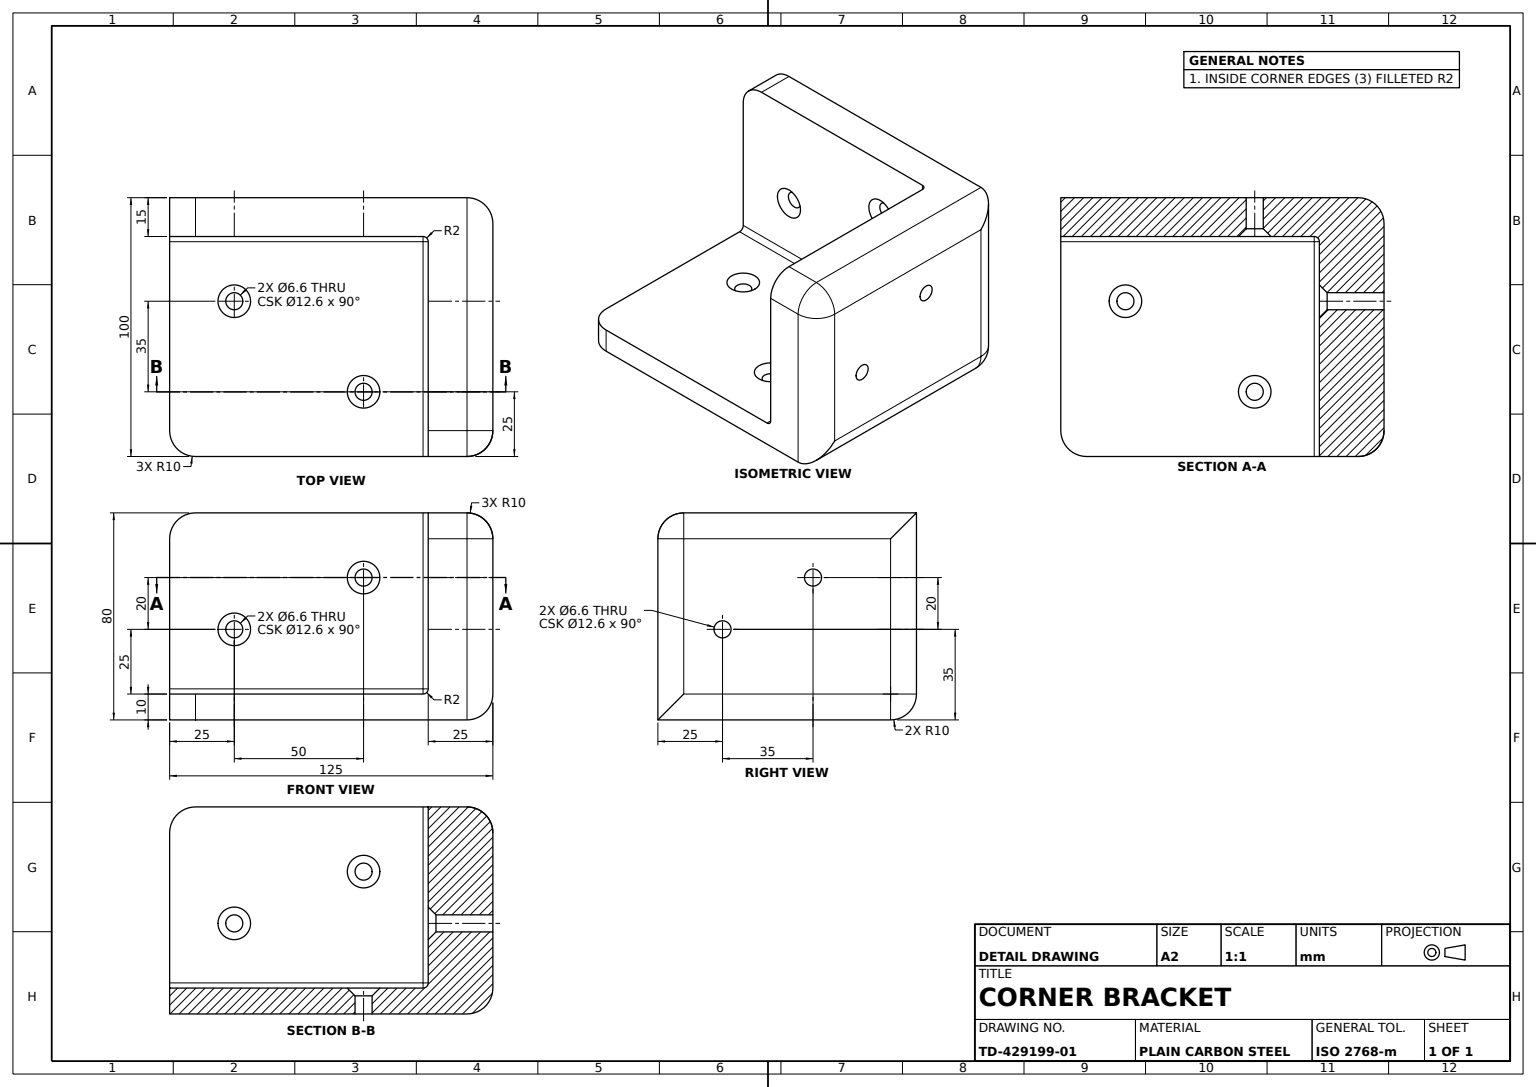
from build123d import *

# Parameters (mm, degrees)
BRACKET_L_PROFILE_SKETCH_W                   = 100
BRACKET_L_PROFILE_SKETCH_H                   = 80
BRACKET_BODY_DEPTH                           = 125
RECTANGULAR_CUT_SKETCH_10X15_W               = 85
RECTANGULAR_CUT_SKETCH_10X15_H               = 70
RECTANGULAR_CUT_10X15_DEPTH                  = 100
COUNTERSUNK_HOLES_6XM6_D                     = 6.6
COUNTERSUNK_HOLES_6XM6_DEPTH                 = 36.017159957
COUNTERSUNK_HOLES_6XM6_CSINK_D               = 12.6
COUNTERSUNK_HOLES_6XM6_CSINK_ANGLE           = 90
COUNTERSUNK_HOLES_6XM6_TIP                   = 1.982840043
COUNTERSUNK_HOLES_6XM6_ON_FACE_2_D           = 6.6
COUNTERSUNK_HOLES_6XM6_ON_FACE_2_DEPTH       = 36.017159957
COUNTERSUNK_HOLES_6XM6_ON_FACE_2_CSINK_D     = 12.6
COUNTERSUNK_HOLES_6XM6_ON_FACE_2_CSINK_ANGLE = 90
COUNTERSUNK_HOLES_6XM6_ON_FACE_2_TIP         = 1.982840043
COUNTERSUNK_HOLES_6XM6_ON_FACE_3_D           = 6.6
COUNTERSUNK_HOLES_6XM6_ON_FACE_3_DEPTH       = 36.017159957
COUNTERSUNK_HOLES_6XM6_ON_FACE_3_CSINK_D     = 12.6
COUNTERSUNK_HOLES_6XM6_ON_FACE_3_CSINK_ANGLE = 90
COUNTERSUNK_HOLES_6XM6_ON_FACE_3_TIP         = 1.982840043
OUTER_EDGE_FILLETS_R10_R                     = 10
EDGE_FILLETS_R2_R                            = 2


with BuildPart() as part:
    # Bracket L-Profile Sketch → Bracket Body (new body)
    with BuildSketch(Plane.XY):
        Rectangle(BRACKET_L_PROFILE_SKETCH_W, BRACKET_L_PROFILE_SKETCH_H)
    extrude(amount=BRACKET_BODY_DEPTH)

    # Rectangular Cut Sketch 10x15 → Rectangular Cut 10x15 (cut)
    with BuildSketch(Plane.XY.offset(125)):
        with Locations((7.5, 5)):
            Rectangle(RECTANGULAR_CUT_SKETCH_10X15_W, RECTANGULAR_CUT_SKETCH_10X15_H)
    extrude(amount=-RECTANGULAR_CUT_10X15_DEPTH, mode=Mode.SUBTRACT)

    # Countersunk Holes 6xM6
    with Locations(Plane(origin=(-35, -5, 100), x_dir=(0, 1, 0), z_dir=(1, 0, 0))):
        with Locations((0, 0), (20, -50)):
            CounterSinkHole(COUNTERSUNK_HOLES_6XM6_D / 2, COUNTERSUNK_HOLES_6XM6_CSINK_D / 2, depth=COUNTERSUNK_HOLES_6XM6_DEPTH, counter_sink_angle=COUNTERSUNK_HOLES_6XM6_CSINK_ANGLE)
            with Locations((0, 0, -(COUNTERSUNK_HOLES_6XM6_DEPTH + COUNTERSUNK_HOLES_6XM6_TIP / 2))):  # 118° drill point
                Cone(0, COUNTERSUNK_HOLES_6XM6_D / 2, COUNTERSUNK_HOLES_6XM6_TIP, mode=Mode.SUBTRACT)

    # Countersunk Holes 6xM6 on face 2
    with Locations(Plane(origin=(-10, -30, 100), x_dir=(0, 0, 1), z_dir=(0, 1, 0))):
        with Locations((0, 0), (-50, 35)):
            CounterSinkHole(COUNTERSUNK_HOLES_6XM6_ON_FACE_2_D / 2, COUNTERSUNK_HOLES_6XM6_ON_FACE_2_CSINK_D / 2, depth=COUNTERSUNK_HOLES_6XM6_ON_FACE_2_DEPTH, counter_sink_angle=COUNTERSUNK_HOLES_6XM6_ON_FACE_2_CSINK_ANGLE)
            with Locations((0, 0, -(COUNTERSUNK_HOLES_6XM6_ON_FACE_2_DEPTH + COUNTERSUNK_HOLES_6XM6_ON_FACE_2_TIP / 2))):  # 118° drill point
                Cone(0, COUNTERSUNK_HOLES_6XM6_ON_FACE_2_D / 2, COUNTERSUNK_HOLES_6XM6_ON_FACE_2_TIP, mode=Mode.SUBTRACT)

    # Countersunk Holes 6xM6 on face 3
    with Locations(Plane(origin=(25, -5, 25), x_dir=(1, 0, 0), z_dir=(0, 0, 1))):
        with Locations((0, 0), (-35, 20)):
            CounterSinkHole(COUNTERSUNK_HOLES_6XM6_ON_FACE_3_D / 2, COUNTERSUNK_HOLES_6XM6_ON_FACE_3_CSINK_D / 2, depth=COUNTERSUNK_HOLES_6XM6_ON_FACE_3_DEPTH, counter_sink_angle=COUNTERSUNK_HOLES_6XM6_ON_FACE_3_CSINK_ANGLE)
            with Locations((0, 0, -(COUNTERSUNK_HOLES_6XM6_ON_FACE_3_DEPTH + COUNTERSUNK_HOLES_6XM6_ON_FACE_3_TIP / 2))):  # 118° drill point
                Cone(0, COUNTERSUNK_HOLES_6XM6_ON_FACE_3_D / 2, COUNTERSUNK_HOLES_6XM6_ON_FACE_3_TIP, mode=Mode.SUBTRACT)

    # Outer Edge Fillets R10
    outer_edge_fillets_r10_edges = [part.edges().sort_by_distance(p)[0] for p in [
        (50, -35, 125),
        (-42.5, 40, 125),
        (50, 40, 12.5),
        (0, 40, 0),
        (50, 0, 0),
        (0, -40, 0),
        (-50, 0, 0),
        (-50, -40, 62.5),
    ]]
    fillet(outer_edge_fillets_r10_edges, radius=OUTER_EDGE_FILLETS_R10_R)

    # Edge Fillets R2
    edge_fillets_r2_edges = [part.edges().sort_by_distance(p)[0] for p in [
        (-35, 5, 25),
        (-35, -30, 75),
        (7.5, -30, 25),
    ]]
    fillet(edge_fillets_r2_edges, radius=EDGE_FILLETS_R2_R)


solid = part.part
